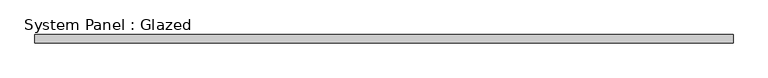
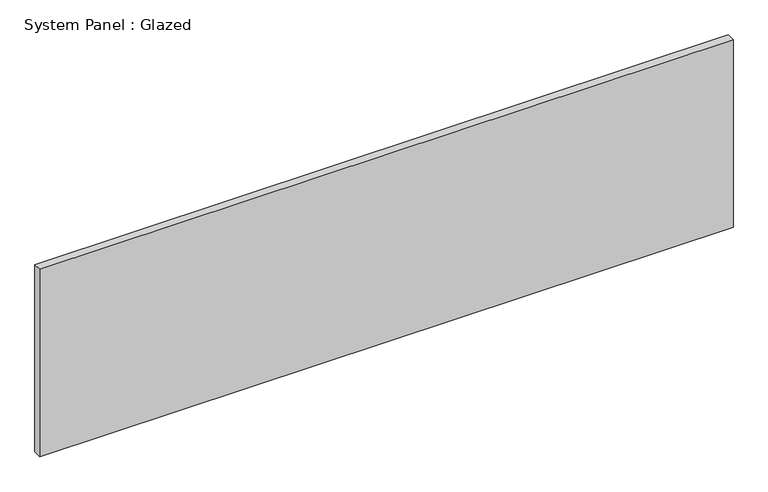
"""IFC4 building model written with IfcOpenShell, lengths in millimetres: plate geometry, System Panel : Glazed."""

from ifc_helpers import new_model, si_unit, origin, origin_with_axes, place, context, project, spatial, polyline, outline, extrude, source, transform, mapped, element, save


def system_panel_glazed_3235cd3f(model_context):
    return source(origin(), model_context, "Body", "SweptSolid", [
        extrude(outline(polyline([(1066.8, 19.05), (-1066.8, 19.05), (-1066.8, 44.45), (1066.8, 44.45), (1066.8, 19.05)])), origin_with_axes(), (0.0, 0.0, 1.0), 609.6),
    ])


if __name__ == "__main__":
    model = new_model("IFC4")
    model_context = context("Model", 3, world=origin())
    ifc_project = project(units=[si_unit("LENGTHUNIT", "METRE", prefix="MILLI")], contexts=[model_context])
    site = spatial("IfcSite", under=ifc_project)
    building = spatial("IfcBuilding", under=site)
    placement = place(None, origin())
    system_panel_glazed_shape = system_panel_glazed_3235cd3f(model_context)
    element("IfcPlate", 1, ObjectType="System Panel : Glazed", at=placement, inside=building, context=model_context, shape_type="MappedRepresentation", body=[
        mapped(system_panel_glazed_shape, transform((0.0, 0.0, 0.0), x_axis=(1.0, 0.0, 0.0), y_axis=(0.0, 1.0, 0.0), z_axis=(0.0, 0.0, 1.0))),
    ])
    save(model, "model.ifc")

# Revit data of these elements
# Type "System Panel : Glazed"
#   Construction Type Id = "GSP4R"
#   Analytic Construction = "1/8 in Pilkington single glazing"
#   Visual Light Transmittance = 0.9
#   Solar Heat Gain Coefficient = 0.86
#   Heat Transfer Coefficient (U) = 1.18115 BTU/(h·ft²·°F)
#   Define Thermal Properties by = 1
# Element 1 (IfcPlate, "System Panel : Glazed")
#   Materials on its faces: "Glass"
# Materials
#   "Glass": class "Glass", colour RGB 0 128 192, transparency 0.75, Description = "Soda Lime Glass", Cost = 0
